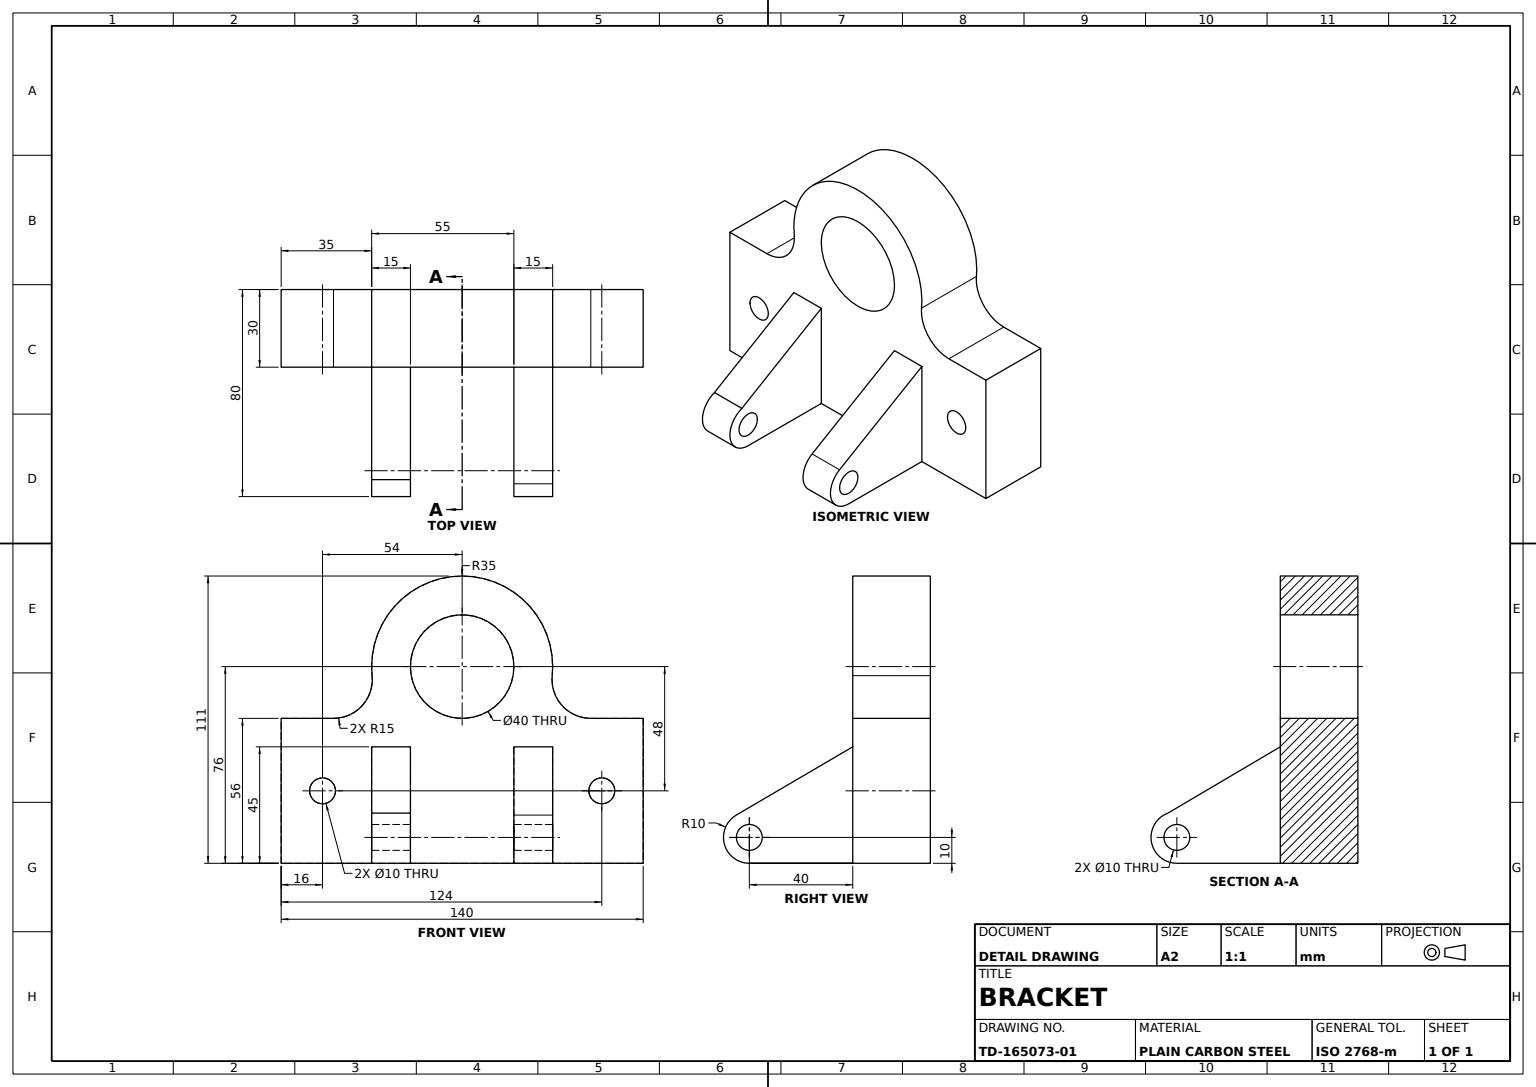
from build123d import *

# Parameters (mm, degrees)
PILLOW_BLOCK_BASE_DEPTH = 15
LUG_ARM_1_DEPTH         = 15
LUG_START               = -15
LUG_ARM_2_DEPTH         = 15
LUG_PIN_HOLE_SKETCH_R   = 5
LUG_PIN_HOLE_DEPTH      = 100
MOUNTING_HOLES_SKETCH_R = 5
MOUNTING_HOLES_2X_DEPTH = 100
SHAFT_BORE_SKETCH_R     = 20
SHAFT_BORE_DEPTH        = 100


with BuildPart() as part:
    # Base Profile Sketch → Pillow Block Base (new, symmetric)
    with BuildSketch(Plane(origin=(0, 0, 0), x_dir=(0, 0, -1), z_dir=(1, 0, 0))):
        with BuildLine():
            Line((0, 0), (-70, 0))
            Line((-70, 0), (-70, 56))
            Line((-70, 56), (-49.749371855, 56))
            ThreePointArc((-49.749371855, 56), (-38.625074125, 60.937694101), (-34.824560299, 72.5))
            ThreePointArc((-34.824560299, 72.5), (0, 111), (34.824560299, 72.5))
            ThreePointArc((34.824560299, 72.5), (38.625074125, 60.937694101), (49.749371855, 56))
            Line((49.749371855, 56), (70, 56))
            Line((70, 56), (70, 0))
            Line((70, 0), (0, 0))
        make_face()
    extrude(amount=PILLOW_BLOCK_BASE_DEPTH, both=True)

    # Lug Arm 1 Sketch → Lug Arm 1 (add)
    with BuildSketch(Plane.XY.offset(20)):
        with BuildLine():
            Line((15, 0), (55, 0))
            ThreePointArc((55, 0), (64.845332755, 8.248023132), (58.449759048, 19.386115411))
            Line((58.449759048, 19.386115411), (15, 45))
            Line((15, 45), (15, 0))
        make_face()
    extrude(amount=LUG_ARM_1_DEPTH)

    # Lug Arm 2 Sketch → Lug Arm 2 (add)
    with BuildSketch(Plane.XY.offset(-20).offset(LUG_START)):
        with BuildLine():
            Line((15, 0), (55, 0))
            ThreePointArc((55, 0), (64.651503897, 7.383041358), (60.051517306, 18.630305493))
            Line((60.051517306, 18.630305493), (15, 45))
            Line((15, 45), (15, 0))
        make_face()
    extrude(amount=LUG_ARM_2_DEPTH)

    # Lug Pin Hole Sketch → Lug Pin Hole (cut)
    with BuildSketch(Plane(origin=(0, 0, -35), x_dir=(-1, 0, 0), z_dir=(0, 0, -1))):
        with Locations((-55, 10)):
            Circle(LUG_PIN_HOLE_SKETCH_R)
    extrude(amount=-LUG_PIN_HOLE_DEPTH, mode=Mode.SUBTRACT)

    # Mounting Holes Sketch → Mounting Holes 2x (cut)
    with BuildSketch(Plane(origin=(15, 0, 0), x_dir=(0, 0, -1), z_dir=(1, 0, 0))):
        with Locations((-54, 28)):
            Circle(MOUNTING_HOLES_SKETCH_R)
        with Locations((54, 28)):
            Circle(MOUNTING_HOLES_SKETCH_R)
    extrude(amount=-MOUNTING_HOLES_2X_DEPTH, mode=Mode.SUBTRACT)

    # Shaft Bore Sketch → Shaft Bore (cut)
    with BuildSketch(Plane(origin=(15, 0, 0), x_dir=(0, 0, -1), z_dir=(1, 0, 0))):
        with Locations((0, 76)):
            Circle(SHAFT_BORE_SKETCH_R)
    extrude(amount=-SHAFT_BORE_DEPTH, mode=Mode.SUBTRACT)


solid = part.part
